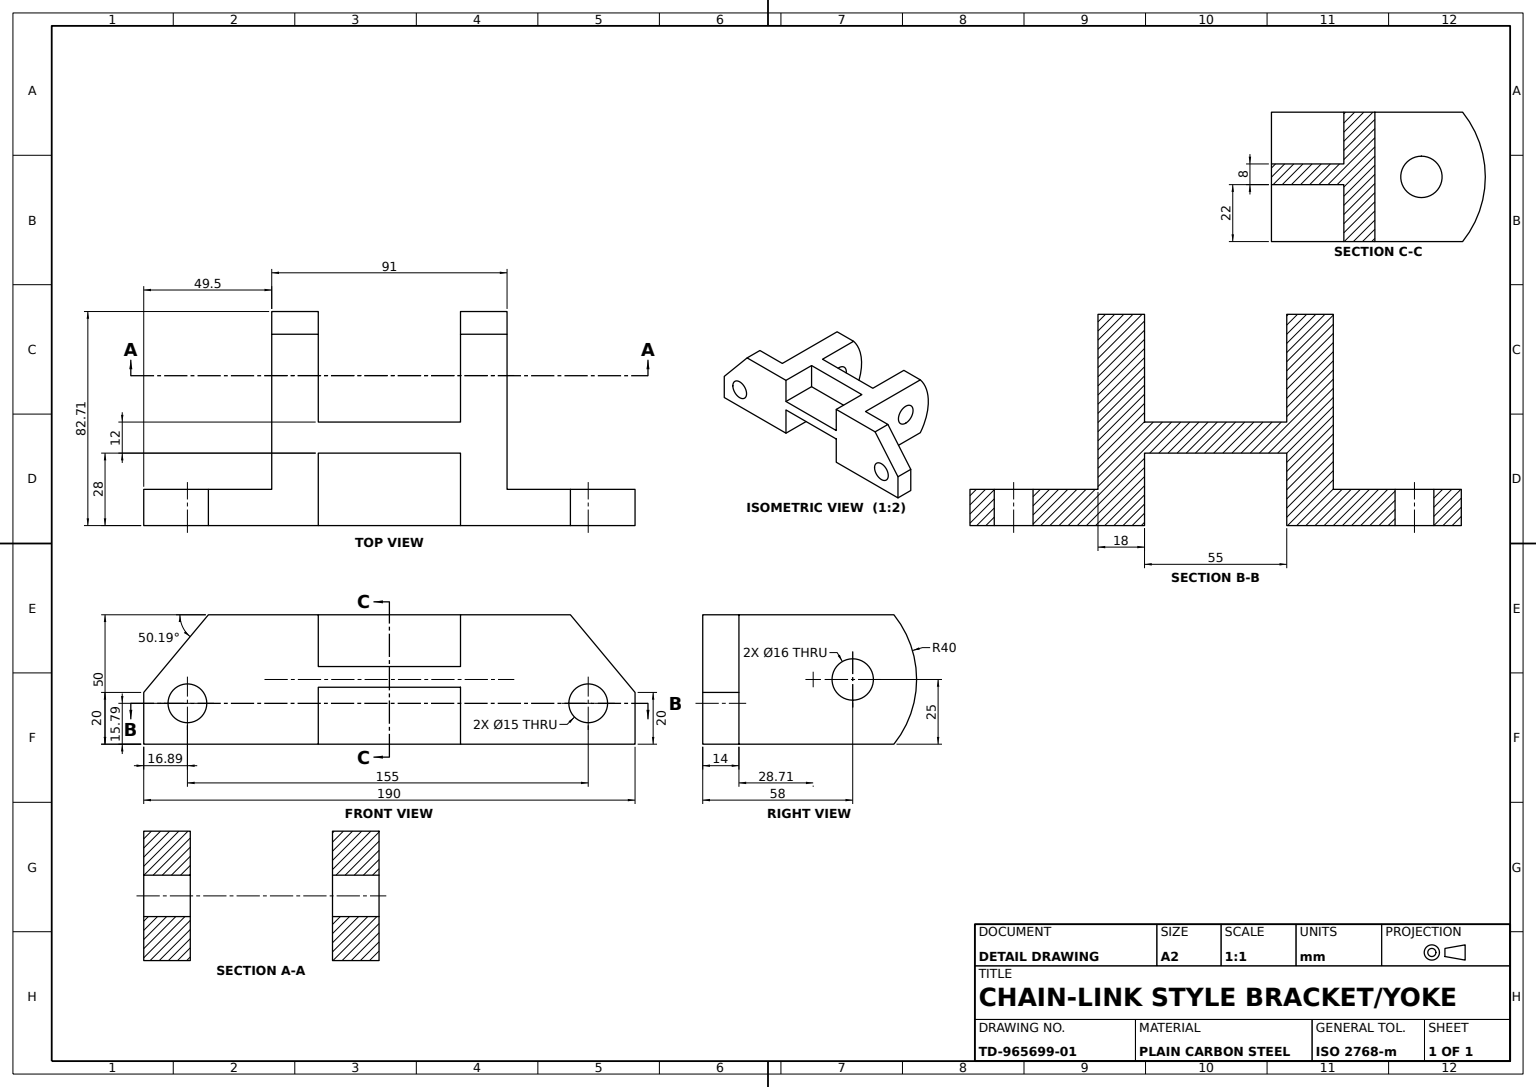
from build123d import *

# Parameters (mm, degrees)
LUG_PLATE_PROFILE_SKETCH_R   = 7.5
LUG_PLATE_PROFILE_14MM_DEPTH = 14
CROSS_BLOCK_SKETCH_W         = 91
CROSS_BLOCK_SKETCH_H         = 84
CROSS_BLOCK_91X84_DEPTH      = 50
CENTRE_POCKET_SKETCH_W       = 55
CENTRE_POCKET_SKETCH_H       = 58
CENTRE_POCKET_55X58_DEPTH    = 50
CLEARANCE_CUT_SKETCH_R       = 8
CLEARANCE_CUT_DEPTH          = 172.161473469
LUG_PIN_HOLES_SKETCH_W       = 55
LUG_PIN_HOLES_SKETCH_H       = 28
LUG_PIN_HOLE_CUT_20MM_DEPTH  = 20
LUG_START                    = -50
SKETCH7_4_W                  = 55
SKETCH7_4_H                  = 28
LUG_PIN_HOLE_CUT_22MM_DEPTH  = 22


with BuildPart() as part:
    # Lug Plate Profile Sketch → Lug Plate Profile 14mm (new body)
    with BuildSketch(Plane.XY):
        Polygon((-94.388010718, 0), (95.611989282, 0), (95.611989282, 20), (70.611989282, 50), (-69.388010718, 50), (-94.388010718, 20), align=None)
        with Locations((-77.5, 15.791749187)):
            Circle(LUG_PLATE_PROFILE_SKETCH_R, mode=Mode.SUBTRACT)
        with Locations((77.5, 15.791749187)):
            Circle(LUG_PLATE_PROFILE_SKETCH_R, mode=Mode.SUBTRACT)
    extrude(amount=LUG_PLATE_PROFILE_14MM_DEPTH)

    # Cross Block Sketch → Cross Block 91x84 (add)
    with BuildSketch(Plane(origin=(0, 50, 0), x_dir=(1, 0, 0), z_dir=(0, 1, 0))):
        with Locations((0.611989282, 42)):
            Rectangle(CROSS_BLOCK_SKETCH_W, CROSS_BLOCK_SKETCH_H)
    extrude(amount=-CROSS_BLOCK_91X84_DEPTH)

    # Centre Pocket Sketch → Centre Pocket 55x58 (cut)
    with BuildSketch(Plane(origin=(0, 50, 0), x_dir=(1, 0, 0), z_dir=(0, 1, 0))):
        with Locations((0.611989282, 55)):
            Rectangle(CENTRE_POCKET_SKETCH_W, CENTRE_POCKET_SKETCH_H)
    extrude(amount=-CENTRE_POCKET_55X58_DEPTH, mode=Mode.SUBTRACT)

    # Clearance Cut Sketch → Clearance Cut (cut, through all)
    with BuildSketch(Plane(origin=(46.111989282, 0, 0), x_dir=(0, 0, -1), z_dir=(1, 0, 0))):
        with Locations(Location((44, 25, 0), (0, 0, 90))):
            Circle(CLEARANCE_CUT_SKETCH_R)
        with BuildLine():
            ThreePointArc((59.934024659, 50), (68.709034667, 25), (59.934024659, 0))
            Line((59.934024659, 0), (84, 0))
            Line((84, 0), (84, 50))
            Line((84, 50), (59.934024659, 50))
        make_face()
    extrude(amount=-CLEARANCE_CUT_DEPTH, mode=Mode.SUBTRACT)

    # Lug Pin Holes Sketch → Lug Pin Hole Cut 20mm (cut)
    with BuildSketch(Plane(origin=(0, 50, 0), x_dir=(1, 0, 0), z_dir=(0, 1, 0))):
        with Locations((0.611989282, 0)):
            Rectangle(LUG_PIN_HOLES_SKETCH_W, LUG_PIN_HOLES_SKETCH_H)
    extrude(amount=-LUG_PIN_HOLE_CUT_20MM_DEPTH, mode=Mode.SUBTRACT)

    # Sketch7_4 → Lug Pin Hole Cut 22mm (cut)
    with BuildSketch(Plane(origin=(0, 50, 0), x_dir=(1, 0, 0), z_dir=(0, 1, 0)).offset(LUG_START)):
        with Locations((0.611989282, 0)):
            Rectangle(SKETCH7_4_W, SKETCH7_4_H)
    extrude(amount=LUG_PIN_HOLE_CUT_22MM_DEPTH, mode=Mode.SUBTRACT)


solid = part.part
